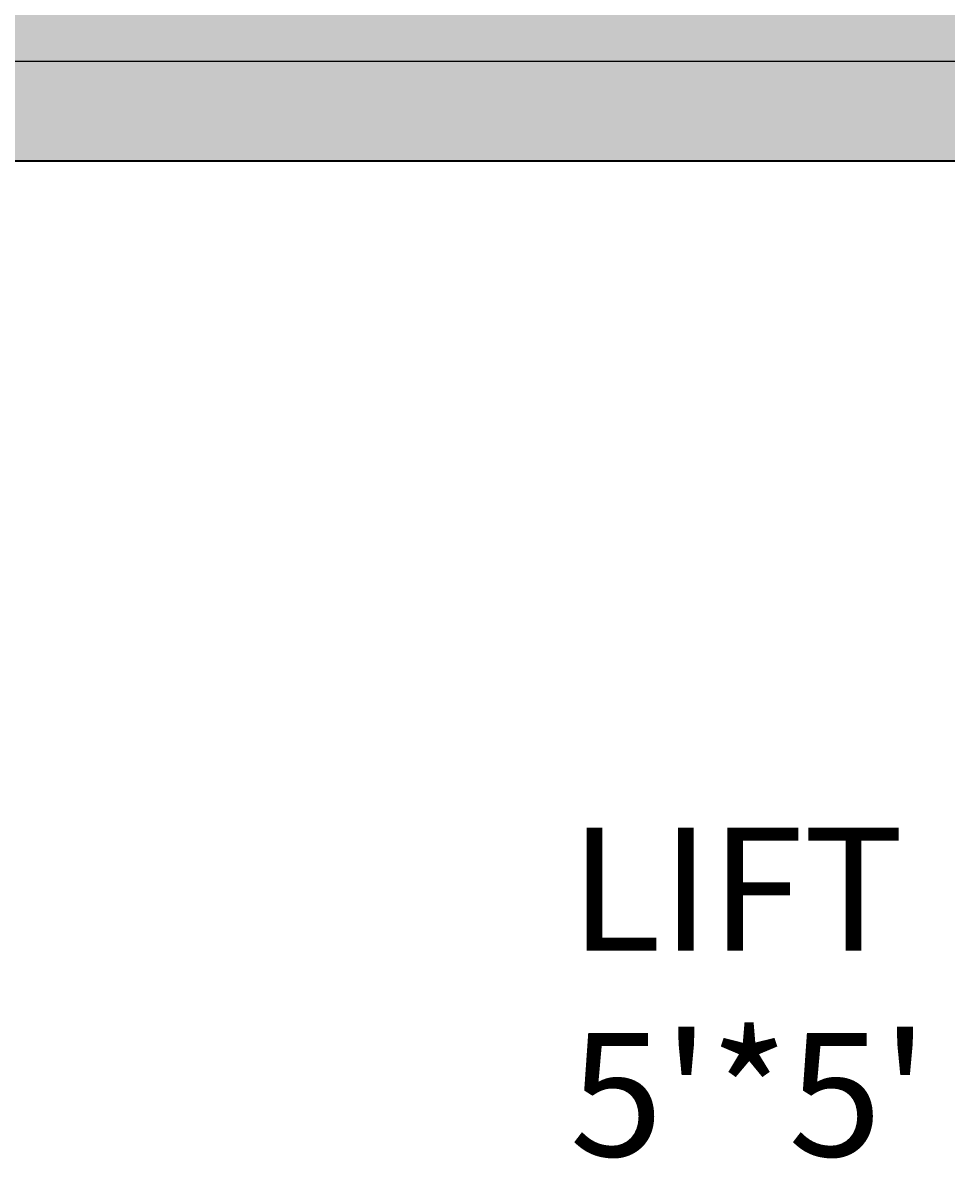
# Model space of a CAD drawing. Units: inches. Extents: x 1998 to 2588, y 1139 to 1977.
# Tile 103 of 134: x 2425 to 2452, y 1555 to 1590. Entities that reach past the tile are written whole.
import ezdxf

# ---------------------------------------------------------------- set-up
doc = ezdxf.new("R2010")
doc.units = ezdxf.units.IN
for name, color, linetype, lineweight in [('A-ANNO-DIMS', 2, 'Continuous', 18), ('A-AREA-IDEN', 7, 'Continuous', 18), ('A-FLOR-EVTR', 7, 'Continuous', 35), ('A-WALL-PATT', 252, 'Continuous', 13)]:
    doc.layers.add(name, color=color, linetype=linetype, lineweight=lineweight)
doc.styles.get("Standard").update_dxf_attribs({"font": 'arial.ttf'})
doc.dimstyles.get("Standard").update_dxf_attribs({"dimtxt": 0.18, "dimasz": 0.18, "dimexe": 0.18, "dimexo": 0.0625, "dimgap": 0.09, "dimtad": 0, "dimtih": 1, "dimtoh": 1, "dimdec": 4, "dimzin": 0, "dimdsep": 46, "dimtxsty": 'Standard', "dimcen": 0.09, "dimadec": 0, "dimazin": 0, "dimtfac": 1, "dimtdec": 4, "dimtofl": 0, "dimtmove": 0, "dimatfit": 3, "dimfxl": 1, "dimtolj": 1, "dimtzin": 0, "dimarcsym": 0})

# ---------------------------------------------------------------- blocks, each defined once
blk = doc.blocks.new('*D24')
at = {"layer": 'A-ANNO-DIMS', "color": 0, "lineweight": -2, "transparency": 16777216}
for p, q in [((2398.535, 1911.232), (2588.309, 1911.232)), ((2588.129, 1911.052), (2588.129, 1570.164)), ((2588.129, 1228.912), (2588.129, 1569.8)), ((2527.535, 1228.732), (2588.309, 1228.732))]:
    blk.add_line(p, q, dxfattribs=at)
at = {"layer": 'A-ANNO-DIMS', "color": 0, "transparency": 16777216}
for points in [[(2588.099, 1911.052), (2588.159, 1911.052), (2588.129, 1911.232)], [(2588.099, 1228.912), (2588.159, 1228.912), (2588.129, 1228.732)]]:
    blk.add_solid(points, dxfattribs=at)
at = {"layer": 'Defpoints', "color": 0, "transparency": 16777216}
for p in [(2398.473, 1911.232), (2588.129, 1911.232), (2527.473, 1228.732)]:
    blk.add_point(p, dxfattribs=at)
at = {"layer": 'A-ANNO-DIMS', "color": 0, "transparency": 16777216, "insert": (2588.129, 1569.982), "char_height": 0.18, "attachment_point": 5}
blk.add_mtext('\\A1;682.5', dxfattribs=at)
blk = doc.blocks.new('*D42')
at = {"layer": 'A-ANNO-DIMS', "color": 0, "lineweight": -2, "transparency": 16777216}
for p, q in [((2287.535, 1588.732), (2588.309, 1588.732)), ((2588.129, 1588.552), (2588.129, 1555.914)), ((2588.129, 1522.912), (2588.129, 1555.55)), ((2287.535, 1522.732), (2588.309, 1522.732))]:
    blk.add_line(p, q, dxfattribs=at)
at = {"layer": 'A-ANNO-DIMS', "color": 0, "transparency": 16777216}
for points in [[(2588.099, 1588.552), (2588.159, 1588.552), (2588.129, 1588.732)], [(2588.099, 1522.912), (2588.159, 1522.912), (2588.129, 1522.732)]]:
    blk.add_solid(points, dxfattribs=at)
at = {"layer": 'Defpoints', "color": 0, "transparency": 16777216}
for p in [(2287.473, 1588.732), (2588.129, 1588.732), (2287.473, 1522.732)]:
    blk.add_point(p, dxfattribs=at)
at = {"layer": 'A-ANNO-DIMS', "color": 0, "transparency": 16777216, "insert": (2588.129, 1555.732), "char_height": 0.18, "attachment_point": 5}
blk.add_mtext('\\A1;66', dxfattribs=at)

msp = doc.modelspace()

# ---------------------------------------------------------------- hatches: boundary and pattern name
at = {"layer": 'A-WALL-PATT'}
h = msp.add_hatch(color=256, dxfattribs=at)
h.dxf.hatch_style = 1
h.paths.add_polyline_path([(2527.4729, 1362.2324), (2510.9729, 1362.2324), (2510.9729, 1357.7324), (2518.4729, 1357.7324), (2518.4729, 1237.7324), (2503.1458, 1237.7324), (2503.1458, 1228.7324), (2527.4729, 1228.7324)])
h.paths.add_polyline_path([(2490.5682, 1362.2324), (2398.4729, 1362.2324), (2398.4729, 1357.7324), (2490.5682, 1357.7324)])
h.paths.add_polyline_path([(2224.9729, 1264.7324), (2222.9729, 1264.7324), (2222.9729, 1232.4125), (2341.4729, 1232.4125), (2341.4729, 1234.4125), (2224.9729, 1234.4125)])
h.paths.add_polyline_path([(2334.5332, 1273.7324), (2264.7638, 1273.7324), (2264.7638, 1269.5611, -0.043659), (2264.3413, 1264.7324), (2334.5332, 1264.7324)])
h.paths.add_polyline_path([(2236.9551, 1273.7324), (2234.4125, 1273.7324), (2234.4125, 1264.7324), (2236.9551, 1264.7324), (2236.9551, 1269.5611)])
h.paths.add_polyline_path([(2222.9729, 1293.2324), (2096.9729, 1293.2324), (2096.9729, 1345.0966), (2087.9729, 1345.0966), (2087.9729, 1284.2324), (2222.9729, 1284.2324), (2222.9729, 1285.137)])
h.paths.add_polyline_path([(2096.9729, 1458.7927), (2087.9729, 1458.7927), (2087.9729, 1417.7324), (2087.9729, 1413.2324), (2096.9729, 1413.2324), (2096.9729, 1417.7324)])
h.paths.add_polyline_path([(2096.9729, 1413.2324), (2087.9729, 1413.2324), (2087.9729, 1365.5012), (2096.9729, 1365.5012), (2096.9729, 1369.3358)])
h.paths.add_polyline_path([(2186.2943, 1417.7324), (2138.6074, 1417.7324), (2096.9729, 1417.7324), (2096.9729, 1413.2324), (2138.6074, 1413.2324), (2186.2943, 1413.2324)])
h.paths.add_polyline_path([(2181.4729, 1465.7324), (2176.9729, 1465.7324), (2176.9729, 1451.6434), (2181.4729, 1451.6434)])
h.paths.add_polyline_path([(2181.4729, 1422.1664), (2176.9729, 1422.1664), (2176.9729, 1417.7324), (2181.4729, 1417.7324)])
h.paths.add_polyline_path([(2063.9729, 1465.7324), (2087.9729, 1465.7324), (2087.9729, 1470.2324), (2059.4729, 1470.2324), (2059.4729, 1413.2324), (2087.9729, 1413.2324), (2087.9729, 1417.7324), (2063.9729, 1417.7324)])
h.paths.add_polyline_path([(2181.4729, 1755.2324), (2176.9729, 1755.2324), (2176.9729, 1748.6798), (2177.0513, 1748.6798), (2181.4729, 1748.6798)])
h.paths.add_polyline_path([(2227.4729, 1707.2324), (2220.4647, 1707.2324), (2220.4647, 1702.7324), (2222.9729, 1702.7324), (2222.9729, 1604.637), (2227.4729, 1604.637)])
h.paths.add_polyline_path([(2114.9729, 1702.7324), (2105.9729, 1702.7324), (2105.9729, 1628.4781, -0.0318759), (2110.1012, 1628.7416), (2114.9729, 1628.7416)])
h.paths.add_polyline_path([(2345.9729, 1739.3278), (2341.4729, 1739.3278), (2341.4729, 1647.5211), (2345.9729, 1647.5211)])
h.paths.add_polyline_path([(2350.6273, 1641.2324), (2345.9729, 1641.2324), (2345.9729, 1636.7324), (2350.6273, 1636.7324), (2350.6273, 1639.8729)])
h.paths.add_polyline_path([(2501.9729, 1641.2324), (2407.9729, 1641.2324), (2392.5005, 1641.2324), (2392.5005, 1639.8729), (2392.5005, 1636.7324), (2501.9729, 1636.7324)])
h.paths.add_polyline_path([(2510.9729, 1755.2324), (2501.9729, 1755.2324), (2501.9729, 1641.2324), (2510.9729, 1641.2324)])
h.paths.add_polyline_path([(2549.1786, 1641.2324), (2522.3775, 1641.2324), (2522.3775, 1636.7324), (2540.1786, 1636.7324), (2540.1786, 1480.7324), (2522.3775, 1480.7324), (2522.3775, 1476.2324), (2549.1786, 1476.2324)])
h.paths.add_polyline_path([(2498.1786, 1594.7324), (2407.9729, 1594.7324), (2407.9729, 1585.7324), (2416.9729, 1585.7324), (2489.1786, 1585.7324), (2489.1786, 1531.7324), (2416.9729, 1531.7324), (2407.9729, 1531.7324), (2407.9729, 1522.7324), (2498.1786, 1522.7324)])
h.paths.add_polyline_path([(2351.6437, 1480.7324), (2345.9729, 1480.7324), (2345.9729, 1476.2324), (2351.6437, 1476.2324), (2351.6437, 1477.5919)])
h.paths.add_polyline_path([(2501.9729, 1480.7324), (2498.1786, 1480.7324), (2407.9729, 1480.7324), (2393.5168, 1480.7324), (2393.5168, 1477.5919), (2393.5168, 1476.2324), (2501.9729, 1476.2324)])

# ---------------------------------------------------------------- linework, layer by layer
at = {"layer": 'A-FLOR-EVTR'}
msp.add_lwpolyline([(2416.9729, 1531.7324), (2489.1786, 1531.7324), (2489.1786, 1585.7324), (2416.9729, 1585.7324)], dxfattribs=at)

# ---------------------------------------------------------------- texts
at = {"layer": 'A-AREA-IDEN', "insert": (2441.0291, 1565.7375), "char_height": 3.69875, "attachment_point": 1}
msp.add_mtext_dynamic_manual_height_columns("LIFT\\P5'*5'", width=110.572713, gutter_width=18.4938, heights=[0], dxfattribs=at)

# ---------------------------------------------------------------- dimensions: what is measured, and where the dimension line sits
at = {"layer": 'A-ANNO-DIMS'}
for base, p1, p2, override, picture, middle in [((2588.1286, 1911.2324), (2527.4729, 1228.7324), (2398.4729, 1911.2324), {"dimdec": 1, "dimlfac": 1, "dimrnd": 0, "dimzin": 0, "dimdsep": 46, "dimlunit": 2}, '*D24', (2588.1286, 1569.9824)), ((2588.1286, 1588.7324), (2287.4729, 1522.7324), (2287.4729, 1588.7324), {"dimdec": 0, "dimlfac": 1, "dimrnd": 0, "dimzin": 0, "dimdsep": 46, "dimlunit": 2}, '*D42', (2588.1286, 1555.7324))]:
    dim = msp.add_linear_dim(base=base, p1=p1, p2=p2, angle=90, dimstyle='Standard', override=override, dxfattribs=at)
    dim.commit()
    dim.dimension.update_dxf_attribs({"geometry": picture, "text_midpoint": middle})

doc.saveas('drawing.dxf')
